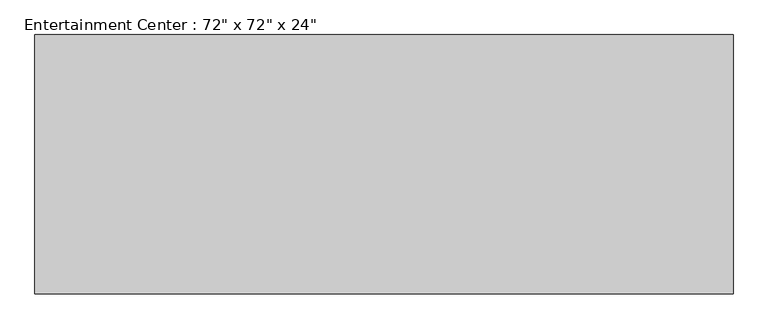
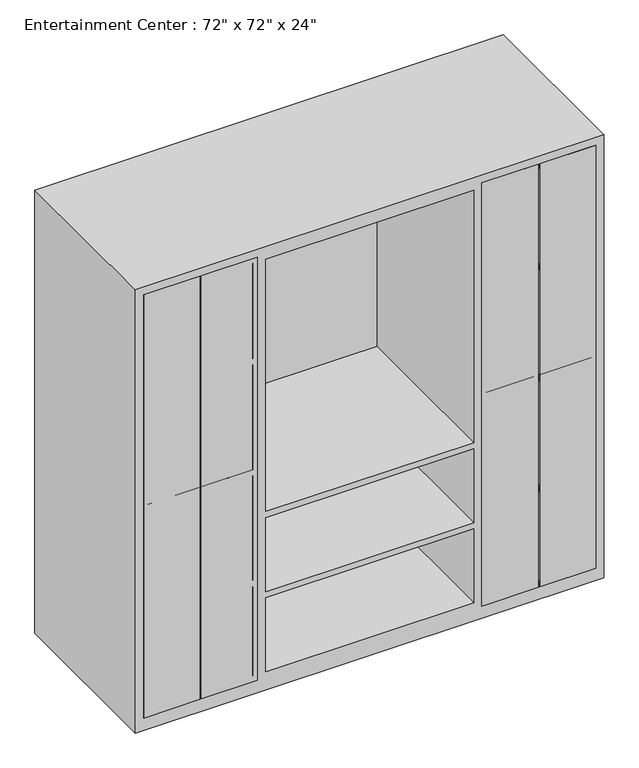
"""IFC4 building model written with IfcOpenShell, lengths in millimetres: furniture geometry."""

from ifc_helpers import new_model, si_unit, point, frame, frame_2d, origin, place, context, project, spatial, polyline, circle_curve, trimmed, segment, composite_curve, outline, extrude, faceted_brep, source, transform, mapped, element, save


def furniture_88072bd9(model_context):
    return source(origin(), model_context, "Body", "SolidModel", [
        extrude(outline(polyline([(-882.65, -711.2), (-663.575, -711.2), (-663.575, -781.05), (-882.65, -781.05), (-882.65, -711.2)])), frame((0.0, 0.0, 50.8), z_axis=(0.0, 0.0, 1.0), x_axis=(1.0, 0.0, 0.0)), (0.0, 0.0, 1.0), 1746.25),
        extrude(outline(polyline([(-657.225, -711.2), (-438.15, -711.2), (-438.15, -781.05), (-657.225, -781.05), (-657.225, -711.2)])), frame((0.0, 0.0, 50.8), z_axis=(0.0, 0.0, 1.0), x_axis=(1.0, 0.0, 0.0)), (0.0, 0.0, 1.0), 1746.25),
        extrude(outline(polyline([(663.575, -711.2), (882.65, -711.2), (882.65, -781.05), (663.575, -781.05), (663.575, -711.2)])), frame((0.0, 0.0, 50.8), z_axis=(0.0, 0.0, 1.0), x_axis=(1.0, 0.0, 0.0)), (0.0, 0.0, 1.0), 1746.25),
        extrude(outline(polyline([(438.15, -711.2), (657.225, -711.2), (657.225, -781.05), (438.15, -781.05), (438.15, -711.2)])), frame((0.0, 0.0, 50.8), z_axis=(0.0, 0.0, 1.0), x_axis=(1.0, 0.0, 0.0)), (0.0, 0.0, 1.0), 1746.25),
        extrude(outline(composite_curve([segment(polyline([(1003.3, -632.9986452), (1003.3, -657.225), (825.5, -657.225), (825.5, -632.9986452)]), True, "CONTINUOUS"), segment(trimmed(circle_curve(frame_2d((850.9, -632.9986452)), 25.4), [point((825.5, -632.9986452))], [point((850.9, -607.5986452))], False, "CARTESIAN"), True, "CONTINUOUS"), segment(polyline([(850.9, -607.5986452), (977.9, -607.5986452)]), True, "CONTINUOUS"), segment(trimmed(circle_curve(frame_2d((977.9, -632.9986452)), 25.4), [point((977.9, -607.5986452))], [point((1003.3, -632.9986452))], False, "CARTESIAN"), True, "CONTINUOUS")], self_intersect=False)), frame((0.0, -714.375, 0.0), z_axis=(0.0, 1.0, 0.0), x_axis=(0.0, 0.0, 1.0)), (0.0, 0.0, 1.0), 3.175),
        extrude(outline(composite_curve([segment(trimmed(circle_curve(frame_2d((977.9, -688.18125)), 25.4), [point((1003.3, -688.18125))], [point((977.9, -713.58125))], False, "CARTESIAN"), True, "CONTINUOUS"), segment(polyline([(977.9, -713.58125), (850.9, -713.58125)]), True, "CONTINUOUS"), segment(trimmed(circle_curve(frame_2d((850.9, -688.18125)), 25.4), [point((850.9, -713.58125))], [point((825.5, -688.18125))], False, "CARTESIAN"), True, "CONTINUOUS"), segment(polyline([(825.5, -688.18125), (825.5, -663.575), (1003.3, -663.575), (1003.3, -688.18125)]), True, "CONTINUOUS")], self_intersect=False)), frame((0.0, -714.375, 0.0), z_axis=(0.0, 1.0, 0.0), x_axis=(0.0, 0.0, 1.0)), (0.0, 0.0, 1.0), 3.175),
        extrude(outline(composite_curve([segment(trimmed(circle_curve(frame_2d((977.9, 632.9986452)), 25.4), [point((1003.3, 632.9986452))], [point((977.9, 607.5986452))], False, "CARTESIAN"), True, "CONTINUOUS"), segment(polyline([(977.9, 607.5986452), (850.9, 607.5986452)]), True, "CONTINUOUS"), segment(trimmed(circle_curve(frame_2d((850.9, 632.9986452)), 25.4), [point((850.9, 607.5986452))], [point((825.5, 632.9986452))], False, "CARTESIAN"), True, "CONTINUOUS"), segment(polyline([(825.5, 632.9986452), (825.5, 657.225), (1003.3, 657.225), (1003.3, 632.9986452)]), True, "CONTINUOUS")], self_intersect=False)), frame((0.0, -714.375, 0.0), z_axis=(0.0, 1.0, 0.0), x_axis=(0.0, 0.0, 1.0)), (0.0, 0.0, 1.0), 3.175),
        extrude(outline(composite_curve([segment(polyline([(1003.3, 688.18125), (1003.3, 663.575), (825.5, 663.575), (825.5, 688.18125)]), True, "CONTINUOUS"), segment(trimmed(circle_curve(frame_2d((850.9, 688.18125)), 25.4), [point((825.5, 688.18125))], [point((850.9, 713.58125))], False, "CARTESIAN"), True, "CONTINUOUS"), segment(polyline([(850.9, 713.58125), (977.9, 713.58125)]), True, "CONTINUOUS"), segment(trimmed(circle_curve(frame_2d((977.9, 688.18125)), 25.4), [point((977.9, 713.58125))], [point((1003.3, 688.18125))], False, "CARTESIAN"), True, "CONTINUOUS")], self_intersect=False)), frame((0.0, -714.375, 0.0), z_axis=(0.0, 1.0, 0.0), x_axis=(0.0, 0.0, 1.0)), (0.0, 0.0, 1.0), 3.175),
        faceted_brep([(914.4, -781.05, 0.0), (914.4, -781.05, 1828.8), (-914.4, -781.05, 1828.8), (-914.4, -781.05, 0.0), (-457.2, -781.05, 1778.0), (-457.2, -781.05, 1384.3), (-863.6, -781.05, 1384.3), (-863.6, -781.05, 1778.0), (-457.2, -781.05, 76.2), (-863.6, -781.05, 76.2), (-863.6, -781.05, 444.5), (-457.2, -781.05, 444.5), (863.6, -781.05, 1384.3), (457.2, -781.05, 1384.3), (457.2, -781.05, 1778.0), (863.6, -781.05, 1778.0), (-406.4, -781.05, 736.6), (-406.4, -781.05, 1778.0), (406.4, -781.05, 1778.0), (406.4, -781.05, 736.6), (406.4, -781.05, 76.2), (-406.4, -781.05, 76.2), (-406.4, -781.05, 381.0), (406.4, -781.05, 381.0), (863.6, -781.05, 76.2), (457.2, -781.05, 76.2), (457.2, -781.05, 444.5), (863.6, -781.05, 444.5), (-863.6, -781.05, 469.9), (-863.6, -781.05, 901.7), (-457.2, -781.05, 901.7), (-457.2, -781.05, 469.9), (-457.2, -781.05, 1358.9), (-457.2, -781.05, 927.1), (-863.6, -781.05, 927.1), (-863.6, -781.05, 1358.9), (457.2, -781.05, 1358.9), (863.6, -781.05, 1358.9), (863.6, -781.05, 927.1), (457.2, -781.05, 927.1), (457.2, -781.05, 901.7), (863.6, -781.05, 901.7), (863.6, -781.05, 469.9), (457.2, -781.05, 469.9), (406.4, -781.05, 406.4), (-406.4, -781.05, 406.4), (-406.4, -781.05, 711.2), (406.4, -781.05, 711.2), (914.4, -101.6, 0.0), (-914.4, -101.6, 0.0), (-914.4, -101.6, 1828.8), (914.4, -101.6, 1828.8), (-457.2, -127.0, 1778.0), (-457.2, -127.0, 1384.3), (-863.6, -127.0, 1384.3), (-863.6, -127.0, 1778.0), (-457.2, -127.0, 76.2), (-863.6, -127.0, 76.2), (-863.6, -127.0, 444.5), (-457.2, -127.0, 444.5), (863.6, -127.0, 1384.3), (457.2, -127.0, 1384.3), (457.2, -127.0, 1778.0), (863.6, -127.0, 1778.0), (-406.4, -127.0, 736.6), (-406.4, -127.0, 1778.0), (406.4, -127.0, 1778.0), (406.4, -127.0, 736.6), (406.4, -127.0, 76.2), (-406.4, -127.0, 76.2), (-406.4, -127.0, 381.0), (406.4, -127.0, 381.0), (863.6, -127.0, 76.2), (457.2, -127.0, 76.2), (457.2, -127.0, 444.5), (863.6, -127.0, 444.5), (-863.6, -127.0, 469.9), (-863.6, -127.0, 901.7), (-457.2, -127.0, 901.7), (-457.2, -127.0, 469.9), (-457.2, -127.0, 1358.9), (-457.2, -127.0, 927.1), (-863.6, -127.0, 927.1), (-863.6, -127.0, 1358.9), (457.2, -127.0, 1358.9), (863.6, -127.0, 1358.9), (863.6, -127.0, 927.1), (457.2, -127.0, 927.1), (457.2, -127.0, 901.7), (863.6, -127.0, 901.7), (863.6, -127.0, 469.9), (457.2, -127.0, 469.9), (406.4, -127.0, 406.4), (-406.4, -127.0, 406.4), (-406.4, -127.0, 711.2), (406.4, -127.0, 711.2)], [[[0, 1, 2, 3], [4, 5, 6, 7], [8, 9, 10, 11], [12, 13, 14, 15], [16, 17, 18, 19], [20, 21, 22, 23], [24, 25, 26, 27], [28, 29, 30, 31], [32, 33, 34, 35], [36, 37, 38, 39], [40, 41, 42, 43], [44, 45, 46, 47]], [[48, 49, 50, 51]], [[1, 0, 48, 51]], [[2, 1, 51, 50]], [[3, 2, 50, 49]], [[0, 3, 49, 48]], [[5, 4, 52, 53]], [[6, 5, 53, 54]], [[7, 6, 54, 55]], [[4, 7, 55, 52]], [[9, 8, 56, 57]], [[10, 9, 57, 58]], [[11, 10, 58, 59]], [[8, 11, 59, 56]], [[13, 12, 60, 61]], [[14, 13, 61, 62]], [[15, 14, 62, 63]], [[12, 15, 63, 60]], [[17, 16, 64, 65]], [[18, 17, 65, 66]], [[19, 18, 66, 67]], [[16, 19, 67, 64]], [[21, 20, 68, 69]], [[22, 21, 69, 70]], [[23, 22, 70, 71]], [[20, 23, 71, 68]], [[25, 24, 72, 73]], [[26, 25, 73, 74]], [[27, 26, 74, 75]], [[24, 27, 75, 72]], [[29, 28, 76, 77]], [[30, 29, 77, 78]], [[31, 30, 78, 79]], [[28, 31, 79, 76]], [[33, 32, 80, 81]], [[34, 33, 81, 82]], [[35, 34, 82, 83]], [[32, 35, 83, 80]], [[37, 36, 84, 85]], [[38, 37, 85, 86]], [[39, 38, 86, 87]], [[36, 39, 87, 84]], [[41, 40, 88, 89]], [[42, 41, 89, 90]], [[43, 42, 90, 91]], [[40, 43, 91, 88]], [[45, 44, 92, 93]], [[46, 45, 93, 94]], [[47, 46, 94, 95]], [[44, 47, 95, 92]], [[53, 52, 55, 54]], [[57, 56, 59, 58]], [[61, 60, 63, 62]], [[65, 64, 67, 66]], [[69, 68, 71, 70]], [[73, 72, 75, 74]], [[77, 76, 79, 78]], [[81, 80, 83, 82]], [[85, 84, 87, 86]], [[89, 88, 91, 90]], [[93, 92, 95, 94]]]),
    ])


if __name__ == "__main__":
    model = new_model("IFC4")
    model_context = context("Model", 3, world=origin())
    ifc_project = project(units=[si_unit("LENGTHUNIT", "METRE", prefix="MILLI")], contexts=[model_context])
    site = spatial("IfcSite", under=ifc_project)
    building = spatial("IfcBuilding", under=site)
    placement = place(None, origin())
    furniture_shape = furniture_88072bd9(model_context)
    element("IfcFurniture", 1, ObjectType="Entertainment Center : 72\" x 72\" x 24\"", at=placement, inside=building, context=model_context, shape_type="MappedRepresentation", body=[
        mapped(furniture_shape, transform((0.0, 0.0, 0.0), x_axis=(1.0, 0.0, 0.0), y_axis=(0.0, 1.0, 0.0), z_axis=(0.0, 0.0, 1.0))),
    ])
    save(model, "model.ifc")

# Revit data of these elements
# Type "Entertainment Center : 72\" x 72\" x 24\""
#   Assembly Code = "E2020200"
#   Center Width = 2' - 8"
#   Depth = 2' - 0"
#   Height = 6' - 0"
#   Width = 6' - 0"
#   Material = none
#   Default Elevation = 0
# Element 1 (IfcFurniture, "Entertainment Center : 72\" x 72\" x 24\"")
#   Materials on its faces: "Steel, Chrome Plated", "Glass - Clear, Grey"
# Materials
#   "Steel, Chrome Plated": class "Metal", colour RGB 17 17 17, transparency 0, Description = "Chromiuim plated steel", Cost = 0
#   "Glass - Clear, Grey": class "Glass", colour RGB 252 255 255, transparency 0.64
